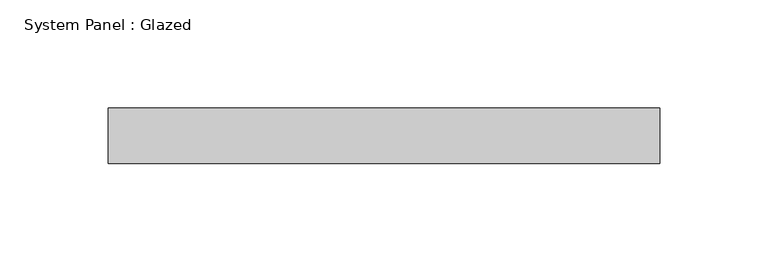
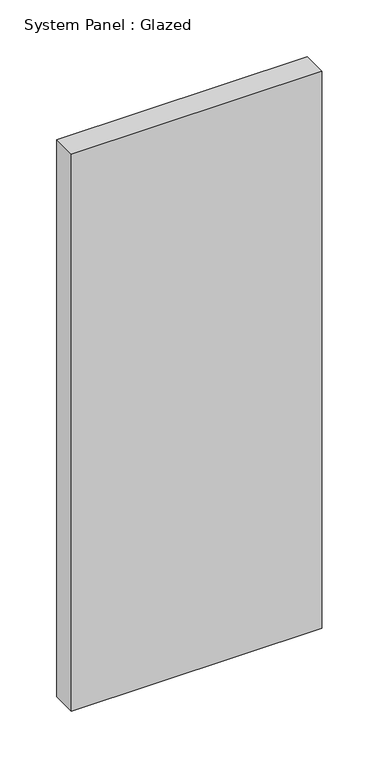
"""IFC4 building model written with IfcOpenShell, lengths in millimetres: plate geometry, System Panel : Glazed."""

from ifc_helpers import new_model, si_unit, origin, origin_with_axes, place, context, project, spatial, polyline, outline, extrude, source, transform, mapped, element, save


def system_panel_glazed_e489fbe4(model_context):
    return source(origin(), model_context, "Body", "SweptSolid", [
        extrude(outline(polyline([(127.0, 19.05), (-127.0, 19.05), (-127.0, 44.45), (127.0, 44.45), (127.0, 19.05)])), origin_with_axes(), (0.0, 0.0, 1.0), 597.1857555),
    ])


if __name__ == "__main__":
    model = new_model("IFC4")
    model_context = context("Model", 3, world=origin())
    ifc_project = project(units=[si_unit("LENGTHUNIT", "METRE", prefix="MILLI")], contexts=[model_context])
    site = spatial("IfcSite", under=ifc_project)
    building = spatial("IfcBuilding", under=site)
    placement = place(None, origin())
    system_panel_glazed_shape = system_panel_glazed_e489fbe4(model_context)
    element("IfcPlate", 1, ObjectType="System Panel : Glazed", at=placement, inside=building, context=model_context, shape_type="MappedRepresentation", body=[
        mapped(system_panel_glazed_shape, transform((0.0, 0.0, 0.0), x_axis=(1.0, 0.0, 0.0), y_axis=(0.0, 1.0, 0.0), z_axis=(0.0, 0.0, 1.0))),
    ])
    save(model, "model.ifc")

# Revit data of these elements
# Type "System Panel : Glazed"
#   Construction Type Id = "GSP4R"
#   Analytic Construction = "1/8 in Pilkington single glazing"
#   Visual Light Transmittance = 0.9
#   Solar Heat Gain Coefficient = 0.86
#   Heat Transfer Coefficient (U) = 1.18115 BTU/(h·ft²·°F)
#   Define Thermal Properties by = 1
# Element 1 (IfcPlate, "System Panel : Glazed")
#   Materials on its faces: "Glass"
# Materials
#   "Glass": class "Glass", colour RGB 0 128 192, transparency 0.75, Description = "Soda Lime Glass", Cost = 0
